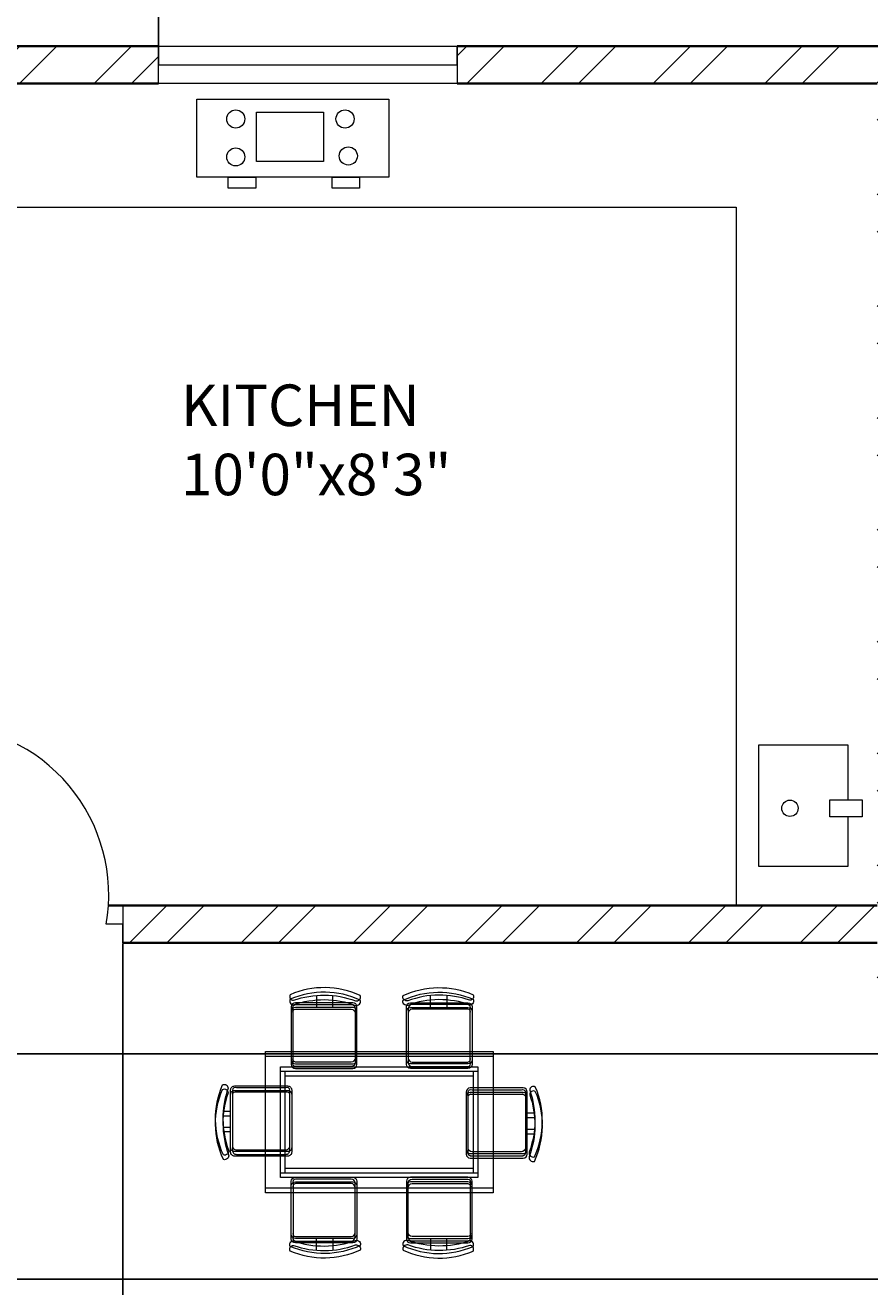
# Model space of a CAD drawing. Units: inches. Extents: x 1965 to 2673, y 1802 to 2669.
# Tile 11 of 16: x 2270 to 2372, y 2416 to 2568. Entities that reach past the tile are written whole.
import ezdxf

# ---------------------------------------------------------------- set-up
doc = ezdxf.new("R2010")
doc.units = ezdxf.units.IN
for name, color, linetype, lineweight in [('A-ANNO-DIMS', 2, 'Continuous', 18), ('A-AREA-IDEN', 7, 'Continuous', 18), ('A-DOOR', 11, 'Continuous', 18), ('A-EQPM', 8, 'Continuous', 18), ('A-FLOR-CASE', 8, 'Continuous', 18), ('A-FLOR-FIXT', 9, 'Continuous', 18), ('A-FURN', 8, 'Continuous', 13), ('A-GLAZ', 181, 'Continuous', 18), ('A-WALL', 7, 'Continuous', 35), ('A-WALL-PATT', 252, 'Continuous', 13)]:
    doc.layers.add(name, color=color, linetype=linetype, lineweight=lineweight)
doc.styles.get("Standard").update_dxf_attribs({"font": 'arial.ttf'})
doc.dimstyles.get("Standard").update_dxf_attribs({"dimtxt": 0.18, "dimasz": 0.18, "dimexe": 0.18, "dimexo": 0.0625, "dimgap": 0.09, "dimtad": 0, "dimtih": 1, "dimtoh": 1, "dimdec": 4, "dimzin": 0, "dimdsep": 46, "dimtxsty": 'Standard', "dimcen": 0.09, "dimadec": 0, "dimazin": 0, "dimtfac": 1, "dimtdec": 4, "dimtofl": 0, "dimtmove": 0, "dimatfit": 3, "dimfxl": 1, "dimtolj": 1, "dimtzin": 0, "dimarcsym": 0})

# ---------------------------------------------------------------- blocks, each defined once
blk = doc.blocks.new('TABLE-DINING-RECT')
for points in [[(0, 16.47), (27.44, 16.47), (27.44, 0), (0, 0)], [(0, 16.47), (27.44, 16.47), (27.44, 0), (0, 0)], [(1.83, 14.64), (25.61, 14.64), (25.61, 1.83), (1.83, 1.83)], [(1.83, 14.64), (25.61, 14.64), (25.61, 1.83), (1.83, 1.83)], [(2.38, 14.09), (25.06, 14.09), (25.06, 2.38), (2.38, 2.38)], [(2.38, 14.09), (25.06, 14.09), (25.06, 2.38), (2.38, 2.38)]]:
    blk.add_lwpolyline(points, close=True)
blk = doc.blocks.new('CHAIR-DINING')
for points in [[(1.58, 0.59, -0.578392), (0.96, 0.02, -0.214524), (0.85, 8.46, -0.552014), (1.52, 8.06, 0.175809), (1.58, 0.59)], [(1.58, 0.59, -0.578392), (0.96, 0.02, -0.214524), (0.85, 8.46, -0.552014), (1.52, 8.06, 0.175809), (1.58, 0.59)], [(1.82, 7.85, -0.414214), (2.31, 8.33), (8.69, 8.33, -0.414214), (9.18, 7.85), (9.18, 0.91, -0.414214), (8.69, 0.42), (2.31, 0.42, -0.414214), (1.82, 0.91), (1.82, 7.85)], [(1.82, 7.85, -0.414214), (2.31, 8.33), (8.69, 8.33, -0.414214), (9.18, 7.85), (9.18, 0.91, -0.414214), (8.69, 0.42), (2.31, 0.42, -0.414214), (1.82, 0.91), (1.82, 7.85)], [(1.82, 3.34), (0.95, 3.34, 0.064759)], [(1.82, 3.34), (0.95, 3.34, 0.064759)]]:
    blk.add_lwpolyline(points, format="xyb")
blk.add_lwpolyline([(2.04, 7.84), (2.04, 1.12, 0.414214), (2.53, 0.64), (8.47, 0.64, 0.414214), (8.96, 1.12), (8.96, 7.84, 0.512069), (8.47, 8.11), (2.53, 8.11, 0.512069)], format="xyb", close=True)
blk.add_lwpolyline([(2.04, 7.84), (2.04, 1.12, 0.414214), (2.53, 0.64), (8.47, 0.64, 0.414214), (8.96, 1.12), (8.96, 7.84, 0.512069), (8.47, 8.11), (2.53, 8.11, 0.512069)], format="xyb", close=True)
blk.add_lwpolyline([(0.93, 5.29), (1.82, 5.29)])
blk.add_lwpolyline([(0.93, 5.29), (1.82, 5.29)])
blk = doc.blocks.new('*D29')
at = {"layer": 'A-ANNO-DIMS', "color": 0, "lineweight": -2, "transparency": 16777216}
for p, q in [((2210.23, 2565.65), (2210.23, 2600.5)), ((2210.41, 2600.32), (2247.71, 2600.32)), ((2285.79, 2600.32), (2248.5, 2600.32)), ((2285.97, 2565.65), (2285.97, 2600.5))]:
    blk.add_line(p, q, dxfattribs=at)
at = {"layer": 'A-ANNO-DIMS', "color": 0, "transparency": 16777216}
for points in [[(2210.41, 2600.35), (2210.41, 2600.29), (2210.23, 2600.32)], [(2285.79, 2600.35), (2285.79, 2600.29), (2285.97, 2600.32)]]:
    blk.add_solid(points, dxfattribs=at)
at = {"layer": 'Defpoints', "color": 0, "transparency": 16777216}
for p in [(2285.97, 2600.32), (2210.23, 2565.59), (2285.97, 2565.59)]:
    blk.add_point(p, dxfattribs=at)
at = {"layer": 'A-ANNO-DIMS', "color": 0, "transparency": 16777216, "insert": (2248.1, 2600.32), "char_height": 0.18, "attachment_point": 5}
blk.add_mtext('\\A1;75.74', dxfattribs=at)
blk = doc.blocks.new('*D30')
at = {"layer": 'A-ANNO-DIMS', "color": 0, "lineweight": -2, "transparency": 16777216}
for p, q in [((2285.97, 2565.65), (2285.97, 2600.5)), ((2286.15, 2600.32), (2337.74, 2600.32)), ((2390.24, 2600.32), (2338.65, 2600.32)), ((2390.42, 2565.65), (2390.42, 2600.5))]:
    blk.add_line(p, q, dxfattribs=at)
at = {"layer": 'A-ANNO-DIMS', "color": 0, "transparency": 16777216}
for points in [[(2286.15, 2600.35), (2286.15, 2600.29), (2285.97, 2600.32)], [(2390.24, 2600.35), (2390.24, 2600.29), (2390.42, 2600.32)]]:
    blk.add_solid(points, dxfattribs=at)
at = {"layer": 'Defpoints', "color": 0, "transparency": 16777216}
for p in [(2390.42, 2600.32), (2285.97, 2565.59), (2390.42, 2565.59)]:
    blk.add_point(p, dxfattribs=at)
at = {"layer": 'A-ANNO-DIMS', "color": 0, "transparency": 16777216, "insert": (2338.2, 2600.32), "char_height": 0.18, "attachment_point": 5}
blk.add_mtext('\\A1;104.44', dxfattribs=at)
blk = doc.blocks.new('*D49')
at = {"layer": 'A-ANNO-DIMS', "color": 0, "lineweight": -2, "transparency": 16777216}
for p, q in [((2573.53, 2444.23), (2012.19, 2444.23)), ((2012.37, 2444.05), (2012.37, 2430.84)), ((2012.37, 2417.27), (2012.37, 2430.48)), ((2573.53, 2417.09), (2012.19, 2417.09))]:
    blk.add_line(p, q, dxfattribs=at)
at = {"layer": 'A-ANNO-DIMS', "color": 0, "transparency": 16777216}
for points in [[(2012.34, 2444.05), (2012.4, 2444.05), (2012.37, 2444.23)], [(2012.34, 2417.27), (2012.4, 2417.27), (2012.37, 2417.09)]]:
    blk.add_solid(points, dxfattribs=at)
at = {"layer": 'Defpoints', "color": 0, "transparency": 16777216}
for p in [(2012.37, 2444.23), (2573.59, 2444.23), (2573.59, 2417.09)]:
    blk.add_point(p, dxfattribs=at)
at = {"layer": 'A-ANNO-DIMS', "color": 0, "transparency": 16777216, "insert": (2012.37, 2430.66), "char_height": 0.18, "attachment_point": 5}
blk.add_mtext('\\A1;27.137', dxfattribs=at)
blk = doc.blocks.new('*D53')
at = {"layer": 'A-ANNO-DIMS', "color": 0, "lineweight": -2, "transparency": 16777216}
for p, q in [((2257.52, 2457.53), (2257.52, 1838.49)), ((2281.66, 2457.53), (2281.66, 1838.49)), ((2257.7, 1838.67), (2269.12, 1838.67)), ((2281.48, 1838.67), (2270.05, 1838.67))]:
    blk.add_line(p, q, dxfattribs=at)
at = {"layer": 'A-ANNO-DIMS', "color": 0, "transparency": 16777216}
for points in [[(2257.7, 1838.7), (2257.7, 1838.64), (2257.52, 1838.67)], [(2281.48, 1838.7), (2281.48, 1838.64), (2281.66, 1838.67)]]:
    blk.add_solid(points, dxfattribs=at)
at = {"layer": 'Defpoints', "color": 0, "transparency": 16777216}
for p in [(2257.52, 2457.59), (2281.66, 2457.59), (2281.66, 1838.67)]:
    blk.add_point(p, dxfattribs=at)
at = {"layer": 'A-ANNO-DIMS', "color": 0, "transparency": 16777216, "insert": (2269.59, 1838.67), "char_height": 0.18, "attachment_point": 5}
blk.add_mtext('\\A1;24.145', dxfattribs=at)

msp = doc.modelspace()

# ---------------------------------------------------------------- hatches: boundary and pattern name
at = {"layer": 'A-WALL-PATT'}
h = msp.add_hatch(dxfattribs=at)
h.set_pattern_fill('ANSI32', color=256)
h.paths.add_polyline_path([(2210.2316, 2563.3414), (2210.2316, 2565.5914), (2136.7559, 2565.5914), (2136.7559, 2561.0914), (2195.5927, 2561.0914), (2195.5927, 2485.8604), (2200.0927, 2485.8604), (2200.0927, 2561.0914), (2210.2316, 2561.0914)])
h.paths.add_polyline_path([(2285.9734, 2565.5914), (2234.2316, 2565.5914), (2234.2316, 2561.0914), (2248.0927, 2561.0914), (2248.0927, 2462.0914), (2200.0927, 2462.0914), (2200.0927, 2465.2357), (2197.8427, 2465.2357), (2195.5927, 2465.2357), (2195.5927, 2457.5914), (2248.0927, 2457.5914), (2248.0927, 2452.628), (2252.5927, 2452.628), (2252.5927, 2457.5914), (2257.5156, 2457.5914), (2257.5156, 2459.8414), (2257.5156, 2462.0914), (2252.5927, 2462.0914), (2252.5927, 2561.0914), (2285.9734, 2561.0914)])
h.paths.add_polyline_path([(2213.1374, 1872.8885), (2461.061, 1872.8885), (2461.061, 1909.9813), (2213.1374, 1909.9813)], flags=9)
h.paths.add_polyline_path([(2328.4056, 1942.3944), (2340.6089, 1942.3944), (2340.6089, 1952.6979), (2328.4056, 1952.6979)], flags=9)
h.paths.add_polyline_path([(2353.5759, 2030.9808), (2376.6455, 2030.9808), (2376.6455, 2041.2844), (2353.5759, 2041.2844)], flags=9)
h.paths.add_polyline_path([(2289.989, 2074.1041), (2326.916, 2074.1041), (2326.916, 2092.7615), (2289.989, 2092.7615)], flags=9)
h.paths.add_polyline_path([(2497.9, 2052.8638), (2548.3741, 2052.8638), (2548.3741, 2071.5212), (2497.9, 2071.5212)], flags=9)
h.paths.add_polyline_path([(2486.59, 2116.4883), (2515.7475, 2116.4883), (2515.7475, 2135.1456), (2486.59, 2135.1456)], flags=9)
h.paths.add_polyline_path([(2497.3007, 2181.2877), (2530.459, 2181.2877), (2530.459, 2199.945), (2497.3007, 2199.945)], flags=9)
h.paths.add_polyline_path([(2288.237, 2190.3228), (2324.1238, 2190.3228), (2324.1238, 2208.9802), (2288.237, 2208.9802)], flags=9)
h.paths.add_polyline_path([(2350.806, 2127.8307), (2387.733, 2127.8307), (2387.733, 2146.488), (2350.806, 2146.488)], flags=9)
h.paths.add_polyline_path([(2530.3237, 2315.2679), (2559.5563, 2315.2679), (2559.5563, 2333.9252), (2530.3237, 2333.9252)], flags=9)
h.paths.add_polyline_path([(2418.419, 2383.4707), (2468.2894, 2383.4707), (2468.2894, 2402.1281), (2418.419, 2402.1281)], flags=9)
h.paths.add_polyline_path([(2327.4503, 2399.0281), (2364.3773, 2399.0281), (2364.3773, 2417.6854), (2327.4503, 2417.6854)], flags=9)
h.paths.add_polyline_path([(2147.9722, 2271.4601), (2197.8426, 2271.4601), (2197.8426, 2290.1174), (2147.9722, 2290.1174)], flags=9)
h.paths.add_polyline_path([(2474.3875, 2421.594), (2524.8616, 2421.594), (2524.8616, 2440.2514), (2474.3875, 2440.2514)], flags=9)
h.paths.add_polyline_path([(2063.9863, 2052.9059), (2114.4604, 2052.9059), (2114.4604, 2071.5632), (2063.9863, 2071.5632)], flags=9)
h.paths.add_polyline_path([(2200.3335, 2133.7067), (2237.2605, 2133.7067), (2237.2605, 2152.364), (2200.3335, 2152.364)], flags=9)
h.paths.add_polyline_path([(2080.5973, 2184.636), (2113.8681, 2184.636), (2113.8681, 2203.2933), (2080.5973, 2203.2933)], flags=9)
h.paths.add_polyline_path([(2102.4918, 2116.4497), (2131.6494, 2116.4497), (2131.6494, 2135.107), (2102.4918, 2135.107)], flags=9)
h.paths.add_polyline_path([(2056.2753, 2308.5576), (2085.5079, 2308.5576), (2085.5079, 2327.2149), (2056.2753, 2327.2149)], flags=9)
h.paths.add_polyline_path([(2385.619, 2500.9729), (2414.8516, 2500.9729), (2414.8516, 2519.6303), (2385.619, 2519.6303)], flags=9)
h.paths.add_polyline_path([(2286.6643, 2508.6826), (2320.0715, 2508.6826), (2320.0715, 2527.34), (2286.6643, 2527.34)], flags=9)
h.paths.add_polyline_path([(2206.5604, 2500.7243), (2235.793, 2500.7243), (2235.793, 2519.3817), (2206.5604, 2519.3817)], flags=25)
h.paths.add_polyline_path([(2062.6644, 2424.4027), (2112.5348, 2424.4027), (2112.5348, 2443.0601), (2062.6644, 2443.0601)], flags=9)
h = msp.add_hatch(dxfattribs=at)
h.set_pattern_fill('ANSI32', color=256)
h.paths.add_polyline_path([(2429.5927, 2468.6101), (2427.3427, 2468.6101), (2425.0927, 2468.6101), (2425.0927, 2462.0914), (2377.0927, 2462.0914), (2377.0927, 2561.0914), (2390.4173, 2561.0914), (2390.4173, 2565.5914), (2321.9734, 2565.5914), (2321.9734, 2561.0914), (2372.5927, 2561.0914), (2372.5927, 2462.0914), (2281.6605, 2462.0914), (2281.6605, 2457.5914), (2372.5927, 2457.5914), (2372.5927, 2451.3316), (2377.0927, 2451.3316), (2377.0927, 2457.5914), (2429.5927, 2457.5914)])
h.paths.add_polyline_path([(2480.8929, 2565.5914), (2414.4173, 2565.5914), (2414.4173, 2561.0914), (2425.0927, 2561.0914), (2425.0927, 2489.9153), (2429.5927, 2489.9153), (2429.5927, 2561.0914), (2480.8929, 2561.0914), (2480.8929, 2563.3414)])
h.paths.add_polyline_path([(2213.1374, 1872.8885), (2461.061, 1872.8885), (2461.061, 1909.9813), (2213.1374, 1909.9813)], flags=9)
h.paths.add_polyline_path([(2328.4056, 1942.3944), (2340.6089, 1942.3944), (2340.6089, 1952.6979), (2328.4056, 1952.6979)], flags=9)
h.paths.add_polyline_path([(2353.5759, 2030.9808), (2376.6455, 2030.9808), (2376.6455, 2041.2844), (2353.5759, 2041.2844)], flags=9)
h.paths.add_polyline_path([(2289.989, 2074.1041), (2326.916, 2074.1041), (2326.916, 2092.7615), (2289.989, 2092.7615)], flags=9)
h.paths.add_polyline_path([(2497.9, 2052.8638), (2548.3741, 2052.8638), (2548.3741, 2071.5212), (2497.9, 2071.5212)], flags=9)
h.paths.add_polyline_path([(2486.59, 2116.4883), (2515.7475, 2116.4883), (2515.7475, 2135.1456), (2486.59, 2135.1456)], flags=9)
h.paths.add_polyline_path([(2497.3007, 2181.2877), (2530.459, 2181.2877), (2530.459, 2199.945), (2497.3007, 2199.945)], flags=9)
h.paths.add_polyline_path([(2288.237, 2190.3228), (2324.1238, 2190.3228), (2324.1238, 2208.9802), (2288.237, 2208.9802)], flags=9)
h.paths.add_polyline_path([(2350.806, 2127.8307), (2387.733, 2127.8307), (2387.733, 2146.488), (2350.806, 2146.488)], flags=9)
h.paths.add_polyline_path([(2530.3237, 2315.2679), (2559.5563, 2315.2679), (2559.5563, 2333.9252), (2530.3237, 2333.9252)], flags=9)
h.paths.add_polyline_path([(2418.419, 2383.4707), (2468.2894, 2383.4707), (2468.2894, 2402.1281), (2418.419, 2402.1281)], flags=9)
h.paths.add_polyline_path([(2327.4503, 2399.0281), (2364.3773, 2399.0281), (2364.3773, 2417.6854), (2327.4503, 2417.6854)], flags=9)
h.paths.add_polyline_path([(2147.9722, 2271.4601), (2197.8426, 2271.4601), (2197.8426, 2290.1174), (2147.9722, 2290.1174)], flags=9)
h.paths.add_polyline_path([(2474.3875, 2421.594), (2524.8616, 2421.594), (2524.8616, 2440.2514), (2474.3875, 2440.2514)], flags=9)
h.paths.add_polyline_path([(2063.9863, 2052.9059), (2114.4604, 2052.9059), (2114.4604, 2071.5632), (2063.9863, 2071.5632)], flags=9)
h.paths.add_polyline_path([(2200.3335, 2133.7067), (2237.2605, 2133.7067), (2237.2605, 2152.364), (2200.3335, 2152.364)], flags=9)
h.paths.add_polyline_path([(2080.5973, 2184.636), (2113.8681, 2184.636), (2113.8681, 2203.2933), (2080.5973, 2203.2933)], flags=9)
h.paths.add_polyline_path([(2102.4918, 2116.4497), (2131.6494, 2116.4497), (2131.6494, 2135.107), (2102.4918, 2135.107)], flags=9)
h.paths.add_polyline_path([(2056.2753, 2308.5576), (2085.5079, 2308.5576), (2085.5079, 2327.2149), (2056.2753, 2327.2149)], flags=9)
h.paths.add_polyline_path([(2385.619, 2500.9729), (2414.8516, 2500.9729), (2414.8516, 2519.6303), (2385.619, 2519.6303)], flags=25)
h.paths.add_polyline_path([(2286.6643, 2508.6826), (2320.0715, 2508.6826), (2320.0715, 2527.34), (2286.6643, 2527.34)], flags=25)
h.paths.add_polyline_path([(2206.5604, 2500.7243), (2235.793, 2500.7243), (2235.793, 2519.3817), (2206.5604, 2519.3817)], flags=9)
h.paths.add_polyline_path([(2062.6644, 2424.4027), (2112.5348, 2424.4027), (2112.5348, 2443.0601), (2062.6644, 2443.0601)], flags=9)

# ---------------------------------------------------------------- linework, layer by layer
at = {"layer": 'A-DOOR'}
for p, q in [((2281.6605, 2462.0914), (2281.6605, 2457.5914)), ((2281.6605, 2459.8414), (2279.6605, 2459.8414)), ((2281.6605, 2457.5914), (2281.6605, 2459.8414))]:
    msp.add_line(p, q, dxfattribs=at)
msp.add_arc((2259.5156, 2463.3869), 20.4545, 350.018178, 90, dxfattribs=at)
at = {"layer": 'A-EQPM'}
for points in [[(2290.5681, 2559.2081), (2313.7156, 2559.2081), (2313.7156, 2549.8404), (2290.5681, 2549.8404)], [(2297.778, 2557.634), (2305.848, 2557.634), (2305.848, 2551.7159), (2297.778, 2551.7159)], [(2294.3791, 2549.8404), (2297.6904, 2549.8404), (2297.6904, 2548.4978), (2294.3791, 2548.4978)], [(2306.8941, 2549.8404), (2310.2054, 2549.8404), (2310.2054, 2548.4978), (2306.8941, 2548.4978)], [(2306.8941, 2549.8404), (2310.2054, 2549.8404), (2310.2054, 2548.4978), (2306.8941, 2548.4978)]]:
    msp.add_lwpolyline(points, close=True, dxfattribs=at)
for centre in [(2295.2769, 2556.8332), (2308.4468, 2556.8332), (2295.2769, 2552.2628), (2308.8376, 2552.38)]:
    msp.add_circle(centre, 1.0938, dxfattribs=at)
at = {"layer": 'A-FLOR-CASE'}
for p, q in [((2252.5927, 2546.2207), (2355.5796, 2546.2207)), ((2355.5796, 2546.2207), (2355.5796, 2462.0914))]:
    msp.add_line(p, q, dxfattribs=at)
at = {"layer": 'A-FLOR-FIXT'}
msp.add_lwpolyline([(2369.0471, 2472.7755), (2369.0471, 2466.8146), (2358.3046, 2466.8146), (2358.3046, 2481.4666), (2369.0471, 2481.4666), (2369.0471, 2474.8157)], dxfattribs=at)
msp.add_lwpolyline([(2366.8493, 2474.8157), (2370.7742, 2474.8157), (2370.7742, 2472.7755), (2366.8493, 2472.7755)], close=True, dxfattribs=at)
msp.add_circle((2362.063, 2473.8179), 0.9853, dxfattribs=at)
at = {"layer": 'A-FURN'}
for points in [[(2302.2388, 2450.6874, -0.17580919), (2309.7143, 2450.6308, 0.57839206), (2310.2806, 2451.2535, 0.21452438), (2301.8424, 2451.3667, 0.55201397), (2302.2388, 2450.6874, -0.06507904)], [(2302.2389, 2450.6871, -0.17580919), (2309.7143, 2450.6305, 0.57839206), (2310.2806, 2451.2532, 0.21452438), (2301.8424, 2451.3664, 0.55201397), (2302.2388, 2450.6871, -0.06507904)], [(2316.0076, 2450.6308, -0.57839206), (2315.4413, 2451.2535, -0.21452438), (2323.8795, 2451.3667, -0.55201397), (2323.4831, 2450.6874, 0.1758092), (2316.0076, 2450.6308)], [(2316.0076, 2450.6305, -0.57839206), (2315.4413, 2451.2532, -0.21452438), (2323.8795, 2451.3664, -0.55201397), (2323.4831, 2450.6871, 0.1758092), (2316.0076, 2450.6305)], [(2302.2388, 2450.1385, -0.17580919), (2309.7143, 2450.0818, 0.57839206), (2310.2806, 2450.7046, 0.21452438), (2301.8424, 2450.8178, 0.55201397), (2302.2388, 2450.1385, -0.06507904)], [(2302.2389, 2450.1382, -0.17580919), (2309.7143, 2450.0816, 0.57839206), (2310.2806, 2450.7043, 0.21452438), (2301.8424, 2450.8175, 0.55201397), (2302.2388, 2450.1382, -0.06507904)], [(2306.9595, 2450.3873), (2306.9595, 2451.265, -0.06475861)], [(2306.9595, 2450.387), (2306.9595, 2451.2647, -0.06475861)], [(2306.9595, 2449.8384), (2306.9595, 2450.7161, -0.06475861)], [(2306.9595, 2449.8381), (2306.9595, 2450.7158, -0.06475861)], [(2316.0076, 2450.0818, -0.57839206), (2315.4413, 2450.7046, -0.21452438), (2323.8795, 2450.8178, -0.55201397), (2323.4831, 2450.1385, 0.1758092), (2316.0076, 2450.0818)], [(2316.0076, 2450.0816, -0.57839206), (2315.4413, 2450.7043, -0.21452438), (2323.8795, 2450.8175, -0.55201397), (2323.4831, 2450.1382, 0.1758092), (2316.0076, 2450.0816)], [(2318.7624, 2450.3873), (2318.7624, 2451.265, 0.06475861)], [(2318.7624, 2450.387), (2318.7624, 2451.2647, 0.06475861)], [(2318.7624, 2449.8384), (2318.7624, 2450.7161, 0.06475861)], [(2318.7624, 2449.8381), (2318.7624, 2450.7158, 0.06475861)], [(2309.3971, 2450.3873), (2302.4572, 2450.3873, 0.41421356), (2301.9717, 2449.9018), (2301.9717, 2443.5207, 0.41421356), (2302.4572, 2443.0351), (2309.3971, 2443.0351, 0.41421356), (2309.8826, 2443.5207), (2309.8826, 2449.9018, 0.41421356), (2309.3971, 2450.3873)], [(2309.3971, 2450.387), (2302.4572, 2450.387, 0.41421356), (2301.9717, 2449.9015), (2301.9717, 2443.5204, 0.41421356), (2302.4572, 2443.0349), (2309.3971, 2443.0349, 0.41421356), (2309.8827, 2443.5204), (2309.8827, 2449.9015, 0.41421356), (2309.3971, 2450.387)], [(2309.3971, 2449.8384), (2302.4572, 2449.8384, 0.41421356), (2301.9717, 2449.3529), (2301.9717, 2442.9718, 0.41421356), (2302.4572, 2442.4862), (2309.3971, 2442.4862, 0.41421356), (2309.8826, 2442.9718), (2309.8826, 2449.3529, 0.41421356), (2309.3971, 2449.8384)], [(2309.3971, 2449.8381), (2302.4572, 2449.8381, 0.41421356), (2301.9717, 2449.3526), (2301.9717, 2442.9715, 0.41421356), (2302.4572, 2442.4859), (2309.3971, 2442.4859, 0.41421356), (2309.8827, 2442.9715), (2309.8827, 2449.3526, 0.41421356), (2309.3971, 2449.8381)], [(2323.2647, 2450.3873, -0.41421356), (2323.7502, 2449.9018), (2323.7502, 2443.5207, -0.41421356), (2323.2647, 2443.0351), (2316.3248, 2443.0351, -0.41421356), (2315.8393, 2443.5207), (2315.8393, 2449.9018, -0.41421356), (2316.3248, 2450.3873), (2323.2647, 2450.3873)], [(2323.2647, 2450.387, -0.41421356), (2323.7503, 2449.9015), (2323.7503, 2443.5204, -0.41421356), (2323.2647, 2443.0349), (2316.3248, 2443.0349, -0.41421356), (2315.8393, 2443.5204), (2315.8393, 2449.9015, -0.41421356), (2316.3248, 2450.387), (2323.2647, 2450.387)], [(2323.2647, 2449.8384, -0.41421356), (2323.7502, 2449.3529), (2323.7502, 2442.9718, -0.41421356), (2323.2647, 2442.4862), (2316.3248, 2442.4862, -0.41421356), (2315.8393, 2442.9718), (2315.8393, 2449.3529, -0.41421356), (2316.3248, 2449.8384), (2323.2647, 2449.8384)], [(2323.2647, 2449.8381, -0.41421356), (2323.7503, 2449.3526), (2323.7503, 2442.9715, -0.41421356), (2323.2647, 2442.4859), (2316.3248, 2442.4859, -0.41421356), (2315.8393, 2442.9715), (2315.8393, 2449.3526, -0.41421356), (2316.3248, 2449.8381), (2323.2647, 2449.8381)], [(2330.399, 2439.6547, 0.41421356), (2329.9134, 2440.1403), (2323.5323, 2440.1403, 0.41421356), (2323.0468, 2439.6547), (2323.0468, 2432.7148, 0.41421356), (2323.5323, 2432.2293), (2329.9134, 2432.2293, 0.41421356), (2330.399, 2432.7148), (2330.399, 2439.6547)], [(2330.399, 2439.6544, 0.41421356), (2329.9135, 2440.14), (2323.5323, 2440.14, 0.41421356), (2323.0468, 2439.6544), (2323.0468, 2432.7145, 0.41421356), (2323.5323, 2432.229), (2329.9135, 2432.229, 0.41421356), (2330.399, 2432.7145), (2330.399, 2439.6544)], [(2330.699, 2439.8731, -0.17580919), (2330.6424, 2432.3976, 0.57839206), (2331.2651, 2431.8313, 0.21452438), (2331.3783, 2440.2695, 0.55201397), (2330.699, 2439.8731, -0.06507904)], [(2330.699, 2439.8728, -0.17580919), (2330.6424, 2432.3974, 0.57839206), (2331.2651, 2431.831, 0.21452438), (2331.3783, 2440.2692, 0.55201397), (2330.699, 2439.8728, -0.06507904)], [(2330.399, 2439.1058, 0.41421356), (2329.9134, 2439.5913), (2323.5323, 2439.5913, 0.41421356), (2323.0468, 2439.1058), (2323.0468, 2432.1659, 0.41421356), (2323.5323, 2431.6804), (2329.9134, 2431.6804, 0.41421356), (2330.399, 2432.1659), (2330.399, 2439.1058)], [(2330.399, 2439.1055, 0.41421356), (2329.9135, 2439.5911), (2323.5323, 2439.5911, 0.41421356), (2323.0468, 2439.1055), (2323.0468, 2432.1656, 0.41421356), (2323.5323, 2431.6801), (2329.9135, 2431.6801, 0.41421356), (2330.399, 2432.1656), (2330.399, 2439.1055)], [(2330.699, 2439.3242, -0.17580919), (2330.6424, 2431.8487, 0.57839206), (2331.2651, 2431.2824, 0.21452438), (2331.3783, 2439.7206, 0.55201397), (2330.699, 2439.3242, -0.06507904)], [(2330.699, 2439.3239, -0.17580919), (2330.6424, 2431.8484, 0.57839206), (2331.2651, 2431.2821, 0.21452438), (2331.3783, 2439.7203, 0.55201397), (2330.699, 2439.3239, -0.06507904)], [(2330.399, 2435.1524), (2331.2767, 2435.1524, -0.06475861)], [(2330.399, 2435.1522), (2331.2767, 2435.1522, -0.06475861)], [(2330.399, 2434.6035), (2331.2767, 2434.6035, -0.06475861)], [(2330.399, 2434.6032), (2331.2767, 2434.6032, -0.06475861)], [(2309.3971, 2422.0216), (2302.4572, 2422.0216, -0.41421356), (2301.9717, 2422.5071), (2301.9717, 2428.8883, -0.41421356), (2302.4572, 2429.3738), (2309.3971, 2429.3738, -0.41421356), (2309.8826, 2428.8883), (2309.8826, 2422.5071, -0.41421356), (2309.3971, 2422.0216)], [(2309.3971, 2422.0213), (2302.4572, 2422.0213, -0.41421356), (2301.9717, 2422.5068), (2301.9717, 2428.888, -0.41421356), (2302.4572, 2429.3735), (2309.3971, 2429.3735, -0.41421356), (2309.8827, 2428.888), (2309.8827, 2422.5068, -0.41421356), (2309.3971, 2422.0213)], [(2309.3971, 2421.4727), (2302.4572, 2421.4727, -0.41421356), (2301.9717, 2421.9582), (2301.9717, 2428.3393, -0.41421356), (2302.4572, 2428.8249), (2309.3971, 2428.8249, -0.41421356), (2309.8826, 2428.3393), (2309.8826, 2421.9582, -0.41421356), (2309.3971, 2421.4727)], [(2309.3971, 2421.4724), (2302.4572, 2421.4724, -0.41421356), (2301.9717, 2421.9579), (2301.9717, 2428.3391, -0.41421356), (2302.4572, 2428.8246), (2309.3971, 2428.8246, -0.41421356), (2309.8827, 2428.3391), (2309.8827, 2421.9579, -0.41421356), (2309.3971, 2421.4724)], [(2323.2647, 2422.0216, 0.41421356), (2323.7502, 2422.5071), (2323.7502, 2428.8883, 0.41421356), (2323.2647, 2429.3738), (2316.3248, 2429.3738, 0.41421356), (2315.8393, 2428.8883), (2315.8393, 2422.5071, 0.41421356), (2316.3248, 2422.0216), (2323.2647, 2422.0216)], [(2323.2647, 2422.0213, 0.41421356), (2323.7503, 2422.5068), (2323.7503, 2428.888, 0.41421356), (2323.2647, 2429.3735), (2316.3248, 2429.3735, 0.41421356), (2315.8393, 2428.888), (2315.8393, 2422.5068, 0.41421356), (2316.3248, 2422.0213), (2323.2647, 2422.0213)], [(2323.2647, 2421.4727, 0.41421356), (2323.7502, 2421.9582), (2323.7502, 2428.3393, 0.41421356), (2323.2647, 2428.8249), (2316.3248, 2428.8249, 0.41421356), (2315.8393, 2428.3393), (2315.8393, 2421.9582, 0.41421356), (2316.3248, 2421.4727), (2323.2647, 2421.4727)], [(2323.2647, 2421.4724, 0.41421356), (2323.7503, 2421.9579), (2323.7503, 2428.3391, 0.41421356), (2323.2647, 2428.8246), (2316.3248, 2428.8246, 0.41421356), (2315.8393, 2428.3391), (2315.8393, 2421.9579, 0.41421356), (2316.3248, 2421.4724), (2323.2647, 2421.4724)], [(2306.9595, 2422.0216), (2306.9595, 2421.1439, 0.06475861)], [(2306.9595, 2422.0213), (2306.9595, 2421.1436, 0.06475861)], [(2318.7624, 2422.0216), (2318.7624, 2421.1439, -0.06475861)], [(2318.7624, 2422.0213), (2318.7624, 2421.1436, -0.06475861)], [(2309.7143, 2421.7782, -0.57839206), (2310.2806, 2421.1555, -0.21452438), (2301.8424, 2421.0422, -0.55201397), (2302.2388, 2421.7216, 0.17580929), (2309.7143, 2421.7782)], [(2309.7143, 2421.7779, -0.57839206), (2310.2806, 2421.1552, -0.21452438), (2301.8424, 2421.0419, -0.55201397), (2302.2388, 2421.7213, 0.17580929), (2309.7143, 2421.7779)], [(2309.7143, 2421.2293, -0.57839206), (2310.2806, 2420.6065, -0.21452438), (2301.8424, 2420.4933, -0.55201397), (2302.2388, 2421.1726, 0.17580929), (2309.7143, 2421.2293)], [(2309.7143, 2421.229, -0.57839206), (2310.2806, 2420.6063, -0.21452438), (2301.8424, 2420.493, -0.55201397), (2302.2388, 2421.1724, 0.17580929), (2309.7143, 2421.229)], [(2306.9595, 2421.4727), (2306.9595, 2420.595, 0.06475861)], [(2306.9595, 2421.4724), (2306.9595, 2420.5947, 0.06475861)], [(2323.4831, 2421.7216, -0.17580928), (2316.0076, 2421.7782, 0.57839206), (2315.4413, 2421.1555, 0.21452438), (2323.8795, 2421.0422, 0.55201397), (2323.4831, 2421.7216, -0.06507904)], [(2323.4831, 2421.1726, -0.17580928), (2316.0076, 2421.2293, 0.57839206), (2315.4413, 2420.6065, 0.21452438), (2323.8795, 2420.4933, 0.55201397), (2323.4831, 2421.1726, -0.06507904)], [(2323.4831, 2421.7213, -0.17580928), (2316.0076, 2421.7779, 0.57839206), (2315.4413, 2421.1552, 0.21452438), (2323.8795, 2421.0419, 0.55201397), (2323.4831, 2421.7213, -0.06507904)], [(2323.4831, 2421.1724, -0.17580928), (2316.0076, 2421.229, 0.57839206), (2315.4413, 2420.6063, 0.21452438), (2323.8795, 2420.493, 0.55201397), (2323.4831, 2421.1724, -0.06507904)], [(2318.7624, 2421.4727), (2318.7624, 2420.595, -0.06475861)], [(2318.7624, 2421.4724), (2318.7624, 2420.5947, -0.06475861)]]:
    msp.add_lwpolyline(points, format="xyb", dxfattribs=at)
for points in [[(2305.0169, 2451.281), (2305.0169, 2450.3873)], [(2305.0169, 2451.2807), (2305.0169, 2450.387)], [(2305.0169, 2450.7321), (2305.0169, 2449.8384)], [(2305.0169, 2450.7318), (2305.0169, 2449.8381)], [(2320.705, 2451.281), (2320.705, 2450.3873)], [(2320.705, 2451.2807), (2320.705, 2450.387)], [(2320.705, 2450.7321), (2320.705, 2449.8384)], [(2320.705, 2450.7318), (2320.705, 2449.8381)], [(2331.2926, 2437.095), (2330.399, 2437.095)], [(2331.2926, 2437.0948), (2330.399, 2437.0948)], [(2331.2926, 2436.5461), (2330.399, 2436.5461)], [(2331.2926, 2436.5458), (2330.399, 2436.5458)], [(2305.0169, 2421.128), (2305.0169, 2422.0216)], [(2305.0169, 2421.1277), (2305.0169, 2422.0213)], [(2320.705, 2421.128), (2320.705, 2422.0216)], [(2320.705, 2421.1277), (2320.705, 2422.0213)], [(2305.0169, 2420.579), (2305.0169, 2421.4727)], [(2305.0169, 2420.5787), (2305.0169, 2421.4724)], [(2320.705, 2420.579), (2320.705, 2421.4727)], [(2320.705, 2420.5787), (2320.705, 2421.4724)]]:
    msp.add_lwpolyline(points, dxfattribs=at)
for points in [[(2302.4601, 2450.1686), (2309.1784, 2450.1686, -0.41421356), (2309.6639, 2449.6831), (2309.6639, 2443.7394, -0.41421356), (2309.1784, 2443.2539), (2302.4601, 2443.2539, -0.51206948), (2302.1904, 2443.7394), (2302.1904, 2449.6831, -0.51206948)], [(2302.4601, 2450.1683), (2309.1784, 2450.1683, -0.41421356), (2309.6639, 2449.6828), (2309.6639, 2443.7391, -0.41421356), (2309.1784, 2443.2536), (2302.4601, 2443.2536, -0.51206948), (2302.1904, 2443.7391), (2302.1904, 2449.6828, -0.51206948)], [(2302.4601, 2449.6197), (2309.1784, 2449.6197, -0.41421356), (2309.6639, 2449.1342), (2309.6639, 2443.1905, -0.41421356), (2309.1784, 2442.705), (2302.4601, 2442.705, -0.51206948), (2302.1904, 2443.1905), (2302.1904, 2449.1342, -0.51206948)], [(2302.4601, 2449.6194), (2309.1784, 2449.6194, -0.41421356), (2309.6639, 2449.1339), (2309.6639, 2443.1902, -0.41421356), (2309.1784, 2442.7047), (2302.4601, 2442.7047, -0.51206948), (2302.1904, 2443.1902), (2302.1904, 2449.1339, -0.51206948)], [(2323.2618, 2450.1686), (2316.5435, 2450.1686, 0.41421356), (2316.058, 2449.6831), (2316.058, 2443.7394, 0.41421356), (2316.5435, 2443.2539), (2323.2618, 2443.2539, 0.51206948), (2323.5315, 2443.7394), (2323.5315, 2449.6831, 0.51206948)], [(2323.2618, 2450.1683), (2316.5435, 2450.1683, 0.41421356), (2316.058, 2449.6828), (2316.058, 2443.7391, 0.41421356), (2316.5435, 2443.2536), (2323.2618, 2443.2536, 0.51206948), (2323.5315, 2443.7391), (2323.5315, 2449.6828, 0.51206948)], [(2323.2618, 2449.6197), (2316.5435, 2449.6197, 0.41421356), (2316.058, 2449.1342), (2316.058, 2443.1905, 0.41421356), (2316.5435, 2442.705), (2323.2618, 2442.705, 0.51206948), (2323.5315, 2443.1905), (2323.5315, 2449.1342, 0.51206948)], [(2323.2618, 2449.6194), (2316.5435, 2449.6194, 0.41421356), (2316.058, 2449.1339), (2316.058, 2443.1902, 0.41421356), (2316.5435, 2442.7047), (2323.2618, 2442.7047, 0.51206948), (2323.5315, 2443.1902), (2323.5315, 2449.1339, 0.51206948)], [(2330.1802, 2439.6518), (2330.1802, 2432.9335, -0.41421356), (2329.6947, 2432.448), (2323.751, 2432.448, -0.41421356), (2323.2655, 2432.9335), (2323.2655, 2439.6518, -0.51206948), (2323.751, 2439.9215), (2329.6947, 2439.9215, -0.51206948)], [(2330.1803, 2439.6515), (2330.1803, 2432.9332, -0.41421356), (2329.6947, 2432.4477), (2323.751, 2432.4477, -0.41421356), (2323.2655, 2432.9332), (2323.2655, 2439.6515, -0.51206948), (2323.751, 2439.9212), (2329.6947, 2439.9212, -0.51206948)], [(2330.1802, 2439.1029), (2330.1802, 2432.3846, -0.41421356), (2329.6947, 2431.8991), (2323.751, 2431.8991, -0.41421356), (2323.2655, 2432.3846), (2323.2655, 2439.1029, -0.51206948), (2323.751, 2439.3726), (2329.6947, 2439.3726, -0.51206948)], [(2330.1803, 2439.1026), (2330.1803, 2432.3843, -0.41421356), (2329.6947, 2431.8988), (2323.751, 2431.8988, -0.41421356), (2323.2655, 2432.3843), (2323.2655, 2439.1026, -0.51206948), (2323.751, 2439.3723), (2329.6947, 2439.3723, -0.51206948)], [(2302.4601, 2422.2403), (2309.1784, 2422.2403, 0.41421356), (2309.6639, 2422.7258), (2309.6639, 2428.6695, 0.41421356), (2309.1784, 2429.1551), (2302.4601, 2429.1551, 0.51206948), (2302.1904, 2428.6695), (2302.1904, 2422.7258, 0.51206948)], [(2302.4601, 2422.24), (2309.1784, 2422.24, 0.41421356), (2309.6639, 2422.7256), (2309.6639, 2428.6692, 0.41421356), (2309.1784, 2429.1548), (2302.4601, 2429.1548, 0.51206948), (2302.1904, 2428.6692), (2302.1904, 2422.7256, 0.51206948)], [(2302.4601, 2421.6914), (2309.1784, 2421.6914, 0.41421356), (2309.6639, 2422.1769), (2309.6639, 2428.1206, 0.41421356), (2309.1784, 2428.6061), (2302.4601, 2428.6061, 0.51206948), (2302.1904, 2428.1206), (2302.1904, 2422.1769, 0.51206948)], [(2302.4601, 2421.6911), (2309.1784, 2421.6911, 0.41421356), (2309.6639, 2422.1766), (2309.6639, 2428.1203, 0.41421356), (2309.1784, 2428.6059), (2302.4601, 2428.6059, 0.51206948), (2302.1904, 2428.1203), (2302.1904, 2422.1766, 0.51206948)], [(2323.2618, 2422.2403), (2316.5435, 2422.2403, -0.41421356), (2316.058, 2422.7258), (2316.058, 2428.6695, -0.41421356), (2316.5435, 2429.1551), (2323.2618, 2429.1551, -0.51206948), (2323.5315, 2428.6695), (2323.5315, 2422.7258, -0.51206948)], [(2323.2618, 2422.24), (2316.5435, 2422.24, -0.41421356), (2316.058, 2422.7256), (2316.058, 2428.6692, -0.41421356), (2316.5435, 2429.1548), (2323.2618, 2429.1548, -0.51206948), (2323.5315, 2428.6692), (2323.5315, 2422.7256, -0.51206948)], [(2323.2618, 2421.6914), (2316.5435, 2421.6914, -0.41421356), (2316.058, 2422.1769), (2316.058, 2428.1206, -0.41421356), (2316.5435, 2428.6061), (2323.2618, 2428.6061, -0.51206948), (2323.5315, 2428.1206), (2323.5315, 2422.1769, -0.51206948)], [(2323.2618, 2421.6911), (2316.5435, 2421.6911, -0.41421356), (2316.058, 2422.1766), (2316.058, 2428.1203, -0.41421356), (2316.5435, 2428.6059), (2323.2618, 2428.6059, -0.51206948), (2323.5315, 2428.1203), (2323.5315, 2422.1766, -0.51206948)]]:
    msp.add_lwpolyline(points, format="xyb", close=True, dxfattribs=at)
at = {"layer": 'A-GLAZ'}
for p, q in [((2285.9734, 2561.0914), (2285.9734, 2565.5914)), ((2285.9734, 2565.5914), (2285.9734, 2563.3414)), ((2285.9734, 2565.5914), (2321.9734, 2565.5914)), ((2321.9734, 2563.3414), (2321.9734, 2565.5914)), ((2321.9734, 2565.5914), (2321.9734, 2561.0914)), ((2285.9734, 2563.3414), (2321.9734, 2563.3414)), ((2321.9734, 2561.0914), (2285.9734, 2561.0914))]:
    msp.add_line(p, q, dxfattribs=at)
at = {"layer": 'A-WALL'}
for p, q in [((2234.2316, 2565.5914), (2285.9734, 2565.5914)), ((2321.9734, 2565.5914), (2390.4173, 2565.5914)), ((2252.5927, 2561.0914), (2285.9734, 2561.0914)), ((2321.9734, 2561.0914), (2372.5927, 2561.0914)), ((2279.929, 2462.0914), (2372.5927, 2462.0914)), ((2281.6605, 2457.5914), (2372.5927, 2457.5914))]:
    msp.add_line(p, q, dxfattribs=at)

# ---------------------------------------------------------------- block references
at = {"layer": 'A-FURN'}
for name, p in [('TABLE-DINING-RECT', (2298.8471, 2428.0565)), ('TABLE-DINING-RECT', (2298.8471, 2427.5076)), ('CHAIR-DINING', (2292.8371, 2432.0465)), ('CHAIR-DINING', (2292.8371, 2431.4976))]:
    msp.add_blockref(name, p, dxfattribs=at)

# ---------------------------------------------------------------- texts
at = {"layer": 'A-AREA-IDEN', "insert": (2288.6749, 2524.8519), "char_height": 5, "attachment_point": 1}
msp.add_mtext_dynamic_manual_height_columns('KITCHEN\\P10\'0"x8\'3"', width=170.478722, gutter_width=12.5, heights=[0], dxfattribs=at)

# ---------------------------------------------------------------- dimensions: what is measured, and where the dimension line sits
at = {"layer": 'A-ANNO-DIMS'}
for base, p1, p2, override, picture, middle in [((2285.9734, 2600.3164), (2210.2316, 2565.5914), (2285.9734, 2565.5914), {"dimdec": 2, "dimlfac": 1, "dimrnd": 0, "dimzin": 0, "dimdsep": 46, "dimlunit": 2}, '*D29', (2248.1025, 2600.3164)), ((2390.4173, 2600.3164), (2285.9734, 2565.5914), (2390.4173, 2565.5914), {"dimdec": 2, "dimlfac": 1, "dimrnd": 0, "dimzin": 0, "dimdsep": 46, "dimlunit": 2}, '*D30', (2338.1953, 2600.3164)), ((2281.6605, 1838.6715), (2257.5156, 2457.5914), (2281.6605, 2457.5914), {"dimdec": 3, "dimlfac": 1, "dimrnd": 0, "dimzin": 0, "dimdsep": 46, "dimlunit": 2}, '*D53', (2269.588, 1838.6715))]:
    dim = msp.add_linear_dim(base=base, p1=p1, p2=p2, dimstyle='Standard', override=override, dxfattribs=at)
    dim.commit()
    dim.dimension.update_dxf_attribs({"geometry": picture, "text_midpoint": middle})
dim = msp.add_linear_dim(base=(2012.3677, 2444.2286), p1=(2573.5927, 2417.0914), p2=(2573.5927, 2444.2286), angle=90, dimstyle='Standard', override={"dimdec": 3, "dimlfac": 1, "dimrnd": 0, "dimzin": 0, "dimdsep": 46, "dimlunit": 2}, dxfattribs=at)
dim.commit()
dim.dimension.update_dxf_attribs({"geometry": '*D49', "text_midpoint": (2012.3677, 2430.66)})

doc.saveas('drawing.dxf')
